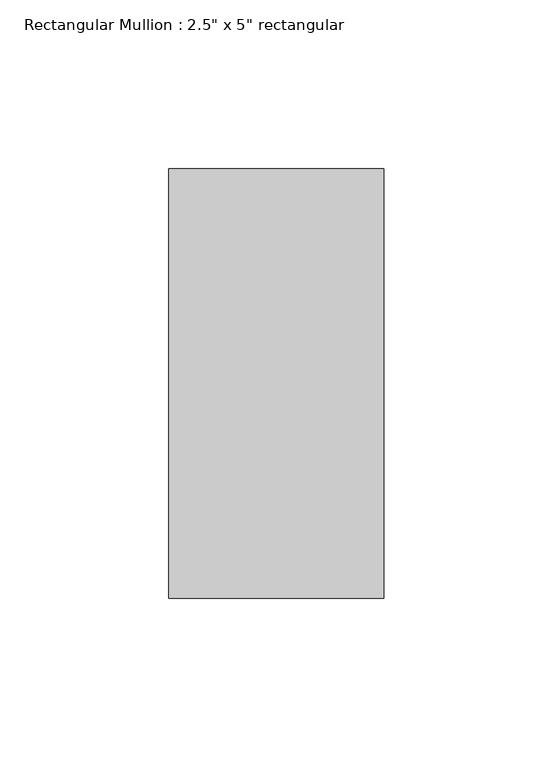
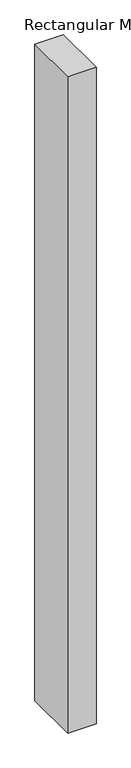
"""IFC4 building model written with IfcOpenShell, lengths in millimetres: member geometry."""

from ifc_helpers import new_model, si_unit, frame, origin, place, context, project, spatial, polyline, outline, extrude, source, transform, mapped, element, save


def member_fff76eb7(model_context):
    return source(origin(), model_context, "Body", "SweptSolid", [
        extrude(outline(polyline([(31.75, 63.5), (31.75, -63.5), (-31.75, -63.5), (-31.75, 63.5), (31.75, 63.5)])), frame((0.0, 0.0, -1551.6345763), z_axis=(0.0, 0.0, 1.0), x_axis=(1.0, 0.0, 0.0)), (0.0, 0.0, 1.0), 1551.6345763),
    ])


if __name__ == "__main__":
    model = new_model("IFC4")
    model_context = context("Model", 3, world=origin())
    ifc_project = project(units=[si_unit("LENGTHUNIT", "METRE", prefix="MILLI")], contexts=[model_context])
    site = spatial("IfcSite", under=ifc_project)
    building = spatial("IfcBuilding", under=site)
    placement = place(None, origin())
    member_shape = member_fff76eb7(model_context)
    element("IfcMember", 1, ObjectType="Rectangular Mullion : 2.5\" x 5\" rectangular", at=placement, inside=building, context=model_context, shape_type="MappedRepresentation", body=[
        mapped(member_shape, transform((0.0, 0.0, 0.0), x_axis=(1.0, 0.0, 0.0), y_axis=(0.0, 1.0, 0.0), z_axis=(0.0, 0.0, 1.0))),
    ])
    save(model, "model.ifc")

# Revit data of these elements
# Type "Rectangular Mullion : 2.5\" x 5\" rectangular"
#   built-in parameter 1007304 = 0.416667 (stored number, unit not read)
#   built-in parameter 1007301 = 0.104167 (stored number, unit not read)
#   built-in parameter 1007300 = 0.104167 (stored number, unit not read)
# Element 1 (IfcMember, "Rectangular Mullion : 2.5\" x 5\" rectangular")
#   Materials on its faces: "Aluminum"
# Materials
#   "Aluminum": class "Metal", colour RGB 247 247 247, transparency 0, Description = "Aluminum 6061", Cost = 0
